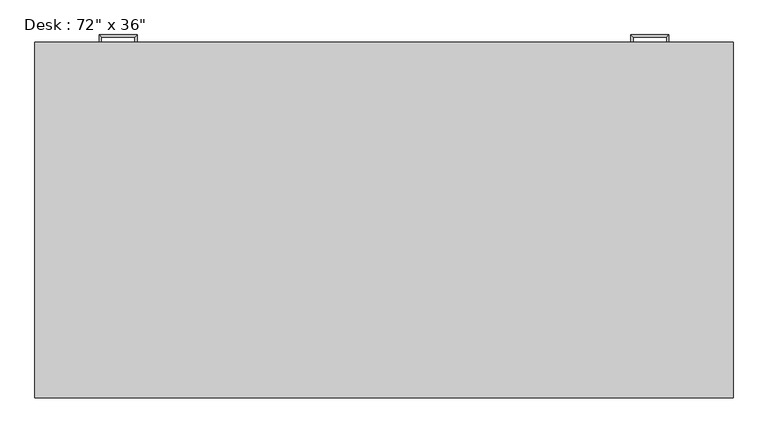
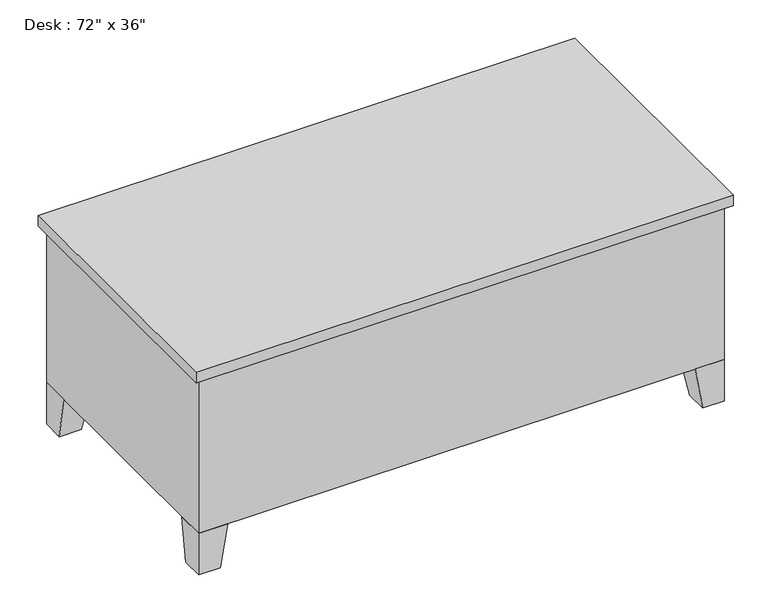
"""IFC4 building model written with IfcOpenShell, lengths in millimetres: furniture geometry."""

from ifc_helpers import new_model, si_unit, frame, origin, place, context, project, spatial, polyline, outline, extrude, faceted_brep, source, transform, mapped, element, save


def furniture_2fc54265(model_context):
    return source(origin(), model_context, "Body", "SolidModel", [
        extrude(outline(polyline([(1809.75, 914.4), (1441.45, 914.4), (1441.45, 927.1), (1809.75, 927.1), (1809.75, 914.4)])), frame((0.0, 0.0, 603.25), z_axis=(0.0, 0.0, 1.0), x_axis=(1.0, 0.0, 0.0)), (0.0, 0.0, 1.0), 101.6),
        extrude(outline(polyline([(1809.75, 914.4), (1441.45, 914.4), (1441.45, 927.1), (1809.75, 927.1), (1809.75, 914.4)])), frame((0.0, 0.0, 171.45), z_axis=(0.0, 0.0, 1.0), x_axis=(1.0, 0.0, 0.0)), (0.0, 0.0, 1.0), 412.75),
        extrude(outline(polyline([(387.35, 914.4), (19.05, 914.4), (19.05, 927.1), (387.35, 927.1), (387.35, 914.4)])), frame((0.0, 0.0, 603.25), z_axis=(0.0, 0.0, 1.0), x_axis=(1.0, 0.0, 0.0)), (0.0, 0.0, 1.0), 101.6),
        extrude(outline(polyline([(387.35, 914.4), (19.05, 914.4), (19.05, 927.1), (387.35, 927.1), (387.35, 914.4)])), frame((0.0, 0.0, 171.45), z_axis=(0.0, 0.0, 1.0), x_axis=(1.0, 0.0, 0.0)), (0.0, 0.0, 1.0), 171.45),
        extrude(outline(polyline([(387.35, 914.4), (19.05, 914.4), (19.05, 927.1), (387.35, 927.1), (387.35, 914.4)])), frame((0.0, 0.0, 482.6), z_axis=(0.0, 0.0, 1.0), x_axis=(1.0, 0.0, 0.0)), (0.0, 0.0, 1.0), 101.6),
        extrude(outline(polyline([(387.35, 914.4), (19.05, 914.4), (19.05, 927.1), (387.35, 927.1), (387.35, 914.4)])), frame((0.0, 0.0, 361.95), z_axis=(0.0, 0.0, 1.0), x_axis=(1.0, 0.0, 0.0)), (0.0, 0.0, 1.0), 101.6),
        faceted_brep([(1727.2, 914.4, 152.4), (1727.2, 812.8, 152.4), (1828.8, 812.8, 152.4), (1828.8, 914.4, 152.4), (1752.6, 914.4, 0.0), (1828.8, 914.4, 0.0), (1828.8, 838.2, 0.0), (1752.6, 838.2, 0.0)], [[[0, 1, 2, 3]], [[4, 5, 6, 7]], [[4, 7, 1, 0]], [[7, 6, 2, 1]], [[6, 5, 3, 2]], [[5, 4, 0, 3]]]),
        faceted_brep([(1727.2, 0.0, 152.4), (1828.8, 0.0, 152.4), (1828.8, 101.6, 152.4), (1727.2, 101.6, 152.4), (1752.6, 0.0, 0.0), (1752.6, 76.2, 0.0), (1828.8, 76.2, 0.0), (1828.8, 0.0, 0.0)], [[[0, 1, 2, 3]], [[4, 5, 6, 7]], [[4, 7, 1, 0]], [[7, 6, 2, 1]], [[6, 5, 3, 2]], [[5, 4, 0, 3]]]),
        faceted_brep([(101.6, 0.0, 152.4), (101.6, 101.6, 152.4), (0.0, 101.6, 152.4), (0.0, 0.0, 152.4), (76.2, 0.0, 0.0), (0.0, 0.0, 0.0), (0.0, 76.2, 0.0), (76.2, 76.2, 0.0)], [[[0, 1, 2, 3]], [[4, 5, 6, 7]], [[4, 7, 1, 0]], [[7, 6, 2, 1]], [[6, 5, 3, 2]], [[5, 4, 0, 3]]]),
        faceted_brep([(101.6, 914.4, 152.4), (0.0, 914.4, 152.4), (0.0, 812.8, 152.4), (101.6, 812.8, 152.4), (76.2, 914.4, 0.0), (76.2, 838.2, 0.0), (0.0, 838.2, 0.0), (0.0, 914.4, 0.0)], [[[0, 1, 2, 3]], [[4, 5, 6, 7]], [[4, 7, 1, 0]], [[7, 6, 2, 1]], [[6, 5, 3, 2]], [[5, 4, 0, 3]]]),
        extrude(outline(polyline([(1847.85, 933.45), (1847.85, -19.05), (-19.05, -19.05), (-19.05, 933.45), (1847.85, 933.45)])), frame((0.0, 0.0, 723.9), z_axis=(0.0, 0.0, 1.0), x_axis=(1.0, 0.0, 0.0)), (0.0, 0.0, 1.0), 38.1),
        extrude(outline(polyline([(406.4, 914.4), (406.4, 50.8), (1422.4, 50.8), (1422.4, 914.4), (1828.8, 914.4), (1828.8, 0.0), (0.0, 0.0), (0.0, 914.4), (406.4, 914.4)])), frame((0.0, 0.0, 152.4), z_axis=(0.0, 0.0, 1.0), x_axis=(1.0, 0.0, 0.0)), (0.0, 0.0, 1.0), 571.5),
        faceted_brep([(1670.05, 927.1, 546.1), (1670.05, 927.1, 533.4), (1676.4, 927.1, 533.4), (1676.4, 927.1, 546.1), (1670.05, 946.15, 546.1), (1670.05, 946.15, 533.4), (1676.4, 952.5, 533.4), (1676.4, 952.5, 546.1), (1581.15, 946.15, 546.1), (1581.15, 946.15, 533.4), (1574.8, 952.5, 533.4), (1574.8, 952.5, 546.1), (1581.15, 927.1, 546.1), (1574.8, 927.1, 546.1), (1574.8, 927.1, 533.4), (1581.15, 927.1, 533.4)], [[[0, 1, 2, 3]], [[1, 0, 4, 5]], [[2, 1, 5, 6]], [[3, 2, 6, 7]], [[0, 3, 7, 4]], [[5, 4, 8, 9]], [[6, 5, 9, 10]], [[7, 6, 10, 11]], [[4, 7, 11, 8]], [[12, 13, 14, 15]], [[9, 8, 12, 15]], [[10, 9, 15, 14]], [[11, 10, 14, 13]], [[8, 11, 13, 12]]]),
        faceted_brep([(1670.05, 927.1, 666.75), (1670.05, 927.1, 654.05), (1676.4, 927.1, 654.05), (1676.4, 927.1, 666.75), (1670.05, 946.15, 666.75), (1670.05, 946.15, 654.05), (1676.4, 952.5, 654.05), (1676.4, 952.5, 666.75), (1581.15, 946.15, 666.75), (1581.15, 946.15, 654.05), (1574.8, 952.5, 654.05), (1574.8, 952.5, 666.75), (1581.15, 927.1, 666.75), (1574.8, 927.1, 666.75), (1574.8, 927.1, 654.05), (1581.15, 927.1, 654.05)], [[[0, 1, 2, 3]], [[1, 0, 4, 5]], [[2, 1, 5, 6]], [[3, 2, 6, 7]], [[0, 3, 7, 4]], [[5, 4, 8, 9]], [[6, 5, 9, 10]], [[7, 6, 10, 11]], [[4, 7, 11, 8]], [[12, 13, 14, 15]], [[9, 8, 12, 15]], [[10, 9, 15, 14]], [[11, 10, 14, 13]], [[8, 11, 13, 12]]]),
        faceted_brep([(158.75, 927.1, 304.8), (152.4, 927.1, 304.8), (152.4, 927.1, 292.1), (158.75, 927.1, 292.1), (158.75, 946.15, 304.8), (152.4, 952.5, 304.8), (152.4, 952.5, 292.1), (158.75, 946.15, 292.1), (247.65, 946.15, 304.8), (254.0, 952.5, 304.8), (254.0, 952.5, 292.1), (247.65, 946.15, 292.1), (247.65, 927.1, 304.8), (247.65, 927.1, 292.1), (254.0, 927.1, 292.1), (254.0, 927.1, 304.8)], [[[0, 1, 2, 3]], [[1, 0, 4, 5]], [[2, 1, 5, 6]], [[3, 2, 6, 7]], [[0, 3, 7, 4]], [[5, 4, 8, 9]], [[6, 5, 9, 10]], [[7, 6, 10, 11]], [[4, 7, 11, 8]], [[12, 13, 14, 15]], [[9, 8, 12, 15]], [[10, 9, 15, 14]], [[11, 10, 14, 13]], [[8, 11, 13, 12]]]),
        faceted_brep([(158.75, 927.1, 425.45), (152.4, 927.1, 425.45), (152.4, 927.1, 412.75), (158.75, 927.1, 412.75), (158.75, 946.15, 425.45), (152.4, 952.5, 425.45), (152.4, 952.5, 412.75), (158.75, 946.15, 412.75), (247.65, 946.15, 425.45), (254.0, 952.5, 425.45), (254.0, 952.5, 412.75), (247.65, 946.15, 412.75), (247.65, 927.1, 425.45), (247.65, 927.1, 412.75), (254.0, 927.1, 412.75), (254.0, 927.1, 425.45)], [[[0, 1, 2, 3]], [[1, 0, 4, 5]], [[2, 1, 5, 6]], [[3, 2, 6, 7]], [[0, 3, 7, 4]], [[5, 4, 8, 9]], [[6, 5, 9, 10]], [[7, 6, 10, 11]], [[4, 7, 11, 8]], [[12, 13, 14, 15]], [[9, 8, 12, 15]], [[10, 9, 15, 14]], [[11, 10, 14, 13]], [[8, 11, 13, 12]]]),
        faceted_brep([(158.75, 927.1, 546.1), (152.4, 927.1, 546.1), (152.4, 927.1, 533.4), (158.75, 927.1, 533.4), (158.75, 946.15, 546.1), (152.4, 952.5, 546.1), (152.4, 952.5, 533.4), (158.75, 946.15, 533.4), (247.65, 946.15, 546.1), (254.0, 952.5, 546.1), (254.0, 952.5, 533.4), (247.65, 946.15, 533.4), (247.65, 927.1, 546.1), (247.65, 927.1, 533.4), (254.0, 927.1, 533.4), (254.0, 927.1, 546.1)], [[[0, 1, 2, 3]], [[1, 0, 4, 5]], [[2, 1, 5, 6]], [[3, 2, 6, 7]], [[0, 3, 7, 4]], [[5, 4, 8, 9]], [[6, 5, 9, 10]], [[7, 6, 10, 11]], [[4, 7, 11, 8]], [[12, 13, 14, 15]], [[9, 8, 12, 15]], [[10, 9, 15, 14]], [[11, 10, 14, 13]], [[8, 11, 13, 12]]]),
        faceted_brep([(158.75, 927.1, 666.75), (152.4, 927.1, 666.75), (152.4, 927.1, 654.05), (158.75, 927.1, 654.05), (158.75, 946.15, 666.75), (152.4, 952.5, 666.75), (152.4, 952.5, 654.05), (158.75, 946.15, 654.05), (247.65, 946.15, 666.75), (254.0, 952.5, 666.75), (254.0, 952.5, 654.05), (247.65, 946.15, 654.05), (247.65, 927.1, 666.75), (247.65, 927.1, 654.05), (254.0, 927.1, 654.05), (254.0, 927.1, 666.75)], [[[0, 1, 2, 3]], [[1, 0, 4, 5]], [[2, 1, 5, 6]], [[3, 2, 6, 7]], [[0, 3, 7, 4]], [[5, 4, 8, 9]], [[6, 5, 9, 10]], [[7, 6, 10, 11]], [[4, 7, 11, 8]], [[12, 13, 14, 15]], [[9, 8, 12, 15]], [[10, 9, 15, 14]], [[11, 10, 14, 13]], [[8, 11, 13, 12]]]),
    ])


if __name__ == "__main__":
    model = new_model("IFC4")
    model_context = context("Model", 3, world=origin())
    ifc_project = project(units=[si_unit("LENGTHUNIT", "METRE", prefix="MILLI")], contexts=[model_context])
    site = spatial("IfcSite", under=ifc_project)
    building = spatial("IfcBuilding", under=site)
    placement = place(None, origin())
    furniture_shape = furniture_2fc54265(model_context)
    element("IfcFurniture", 1, ObjectType="Desk : 72\" x 36\"", at=placement, inside=building, context=model_context, shape_type="MappedRepresentation", body=[
        mapped(furniture_shape, transform((0.0, 0.0, 0.0), x_axis=(1.0, 0.0, 0.0), y_axis=(0.0, 1.0, 0.0), z_axis=(0.0, 0.0, 1.0))),
    ])
    save(model, "model.ifc")

# Revit data of these elements
# Type "Desk : 72\" x 36\""
#   Assembly Code = "E2020200"
#   Depth = 3' - 0"
#   Height = 2' - 6"
#   Leg Height = 0' - 6"
#   Width = 6' - 0"
#   Body Material = Laminate, Ivory, Matte
#   Handle/Leg Material = Steel, Chrome Plated
#   Top Material = Cherry
#   Default Elevation = 0
# Element 1 (IfcFurniture, "Desk : 72\" x 36\"")
#   Materials on its faces: "Steel, Chrome Plated", "Laminate, Ivory, Matte", "Cherry"
# Materials
#   "Laminate, Ivory, Matte": class "Plastic", colour RGB 247 247 239, transparency 0, Description = "Plastic Laminate - Ivory, Matte", Cost = 0
#   "Steel, Chrome Plated": class "Metal", colour RGB 17 17 17, transparency 0, Description = "Chromiuim plated steel", Cost = 0
#   "Cherry": class "Wood", colour RGB 226 177 128, transparency 0, Description = "Prunus Serotina", Cost = 0
